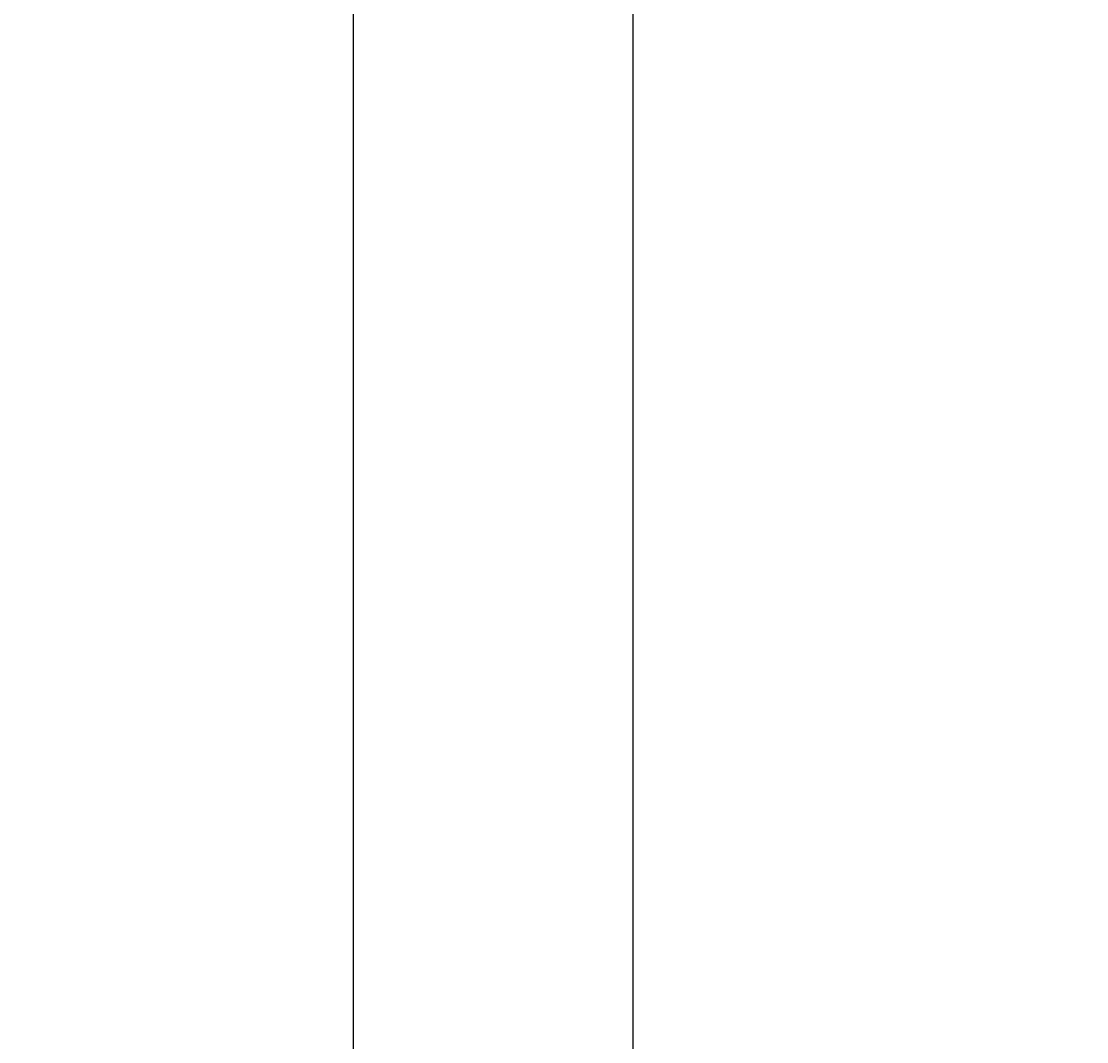
# Model space of a CAD drawing. Units: inches. Extents: x 1998 to 2588, y 1139 to 1977.
# Tile 125 of 134: x 2398 to 2429, y 1669 to 1698. Entities that reach past the tile are written whole.
import ezdxf

# ---------------------------------------------------------------- set-up
doc = ezdxf.new("R2010")
doc.units = ezdxf.units.IN
doc.layers.add('A-ANNO-DIMS', color=2, linetype='Continuous', lineweight=18)
doc.styles.get("Standard").update_dxf_attribs({"font": 'arial.ttf'})
doc.dimstyles.get("Standard").update_dxf_attribs({"dimtxt": 0.18, "dimasz": 0.18, "dimexe": 0.18, "dimexo": 0.0625, "dimgap": 0.09, "dimtad": 0, "dimtih": 1, "dimtoh": 1, "dimdec": 4, "dimzin": 0, "dimdsep": 46, "dimtxsty": 'Standard', "dimcen": 0.09, "dimadec": 0, "dimazin": 0, "dimtfac": 1, "dimtdec": 4, "dimtofl": 0, "dimtmove": 0, "dimatfit": 3, "dimfxl": 1, "dimtolj": 1, "dimtzin": 0, "dimarcsym": 0})

# ---------------------------------------------------------------- blocks, each defined once
blk = doc.blocks.new('*D24')
at = {"layer": 'A-ANNO-DIMS', "color": 0, "lineweight": -2, "transparency": 16777216}
for p, q in [((2398.535, 1911.232), (2588.309, 1911.232)), ((2588.129, 1911.052), (2588.129, 1570.164)), ((2588.129, 1228.912), (2588.129, 1569.8)), ((2527.535, 1228.732), (2588.309, 1228.732))]:
    blk.add_line(p, q, dxfattribs=at)
at = {"layer": 'A-ANNO-DIMS', "color": 0, "transparency": 16777216}
for points in [[(2588.099, 1911.052), (2588.159, 1911.052), (2588.129, 1911.232)], [(2588.099, 1228.912), (2588.159, 1228.912), (2588.129, 1228.732)]]:
    blk.add_solid(points, dxfattribs=at)
at = {"layer": 'Defpoints', "color": 0, "transparency": 16777216}
for p in [(2398.473, 1911.232), (2588.129, 1911.232), (2527.473, 1228.732)]:
    blk.add_point(p, dxfattribs=at)
at = {"layer": 'A-ANNO-DIMS', "color": 0, "transparency": 16777216, "insert": (2588.129, 1569.982), "char_height": 0.18, "attachment_point": 5}
blk.add_mtext('\\A1;682.5', dxfattribs=at)
blk = doc.blocks.new('*D32')
at = {"layer": 'A-ANNO-DIMS', "color": 0, "lineweight": -2, "transparency": 16777216}
for p, q in [((2407.973, 1636.795), (2407.973, 1977.362)), ((2415.973, 1636.795), (2415.973, 1977.362)), ((2408.153, 1977.182), (2411.824, 1977.182)), ((2415.793, 1977.182), (2412.122, 1977.182))]:
    blk.add_line(p, q, dxfattribs=at)
at = {"layer": 'A-ANNO-DIMS', "color": 0, "transparency": 16777216}
for points in [[(2408.153, 1977.212), (2408.153, 1977.152), (2407.973, 1977.182)], [(2415.793, 1977.212), (2415.793, 1977.152), (2415.973, 1977.182)]]:
    blk.add_solid(points, dxfattribs=at)
at = {"layer": 'Defpoints', "color": 0, "transparency": 16777216}
for p in [(2415.973, 1977.182), (2407.973, 1636.732), (2415.973, 1636.732)]:
    blk.add_point(p, dxfattribs=at)
at = {"layer": 'A-ANNO-DIMS', "color": 0, "transparency": 16777216, "insert": (2411.973, 1977.182), "char_height": 0.18, "attachment_point": 5}
blk.add_mtext('\\A1;8', dxfattribs=at)

msp = doc.modelspace()

# ---------------------------------------------------------------- dimensions: what is measured, and where the dimension line sits
at = {"layer": 'A-ANNO-DIMS'}
dim = msp.add_linear_dim(base=(2415.9729, 1977.1824), p1=(2407.9729, 1636.7324), p2=(2415.9729, 1636.7324), dimstyle='Standard', override={"dimdec": 0, "dimlfac": 1, "dimrnd": 0, "dimzin": 0, "dimdsep": 46, "dimlunit": 2}, dxfattribs=at)
dim.commit()
dim.dimension.update_dxf_attribs({"geometry": '*D32', "text_midpoint": (2411.9729, 1977.1824)})
dim = msp.add_linear_dim(base=(2588.1286, 1911.2324), p1=(2527.4729, 1228.7324), p2=(2398.4729, 1911.2324), angle=90, dimstyle='Standard', override={"dimdec": 1, "dimlfac": 1, "dimrnd": 0, "dimzin": 0, "dimdsep": 46, "dimlunit": 2}, dxfattribs=at)
dim.commit()
dim.dimension.update_dxf_attribs({"geometry": '*D24', "text_midpoint": (2588.1286, 1569.9824)})

doc.saveas('drawing.dxf')
